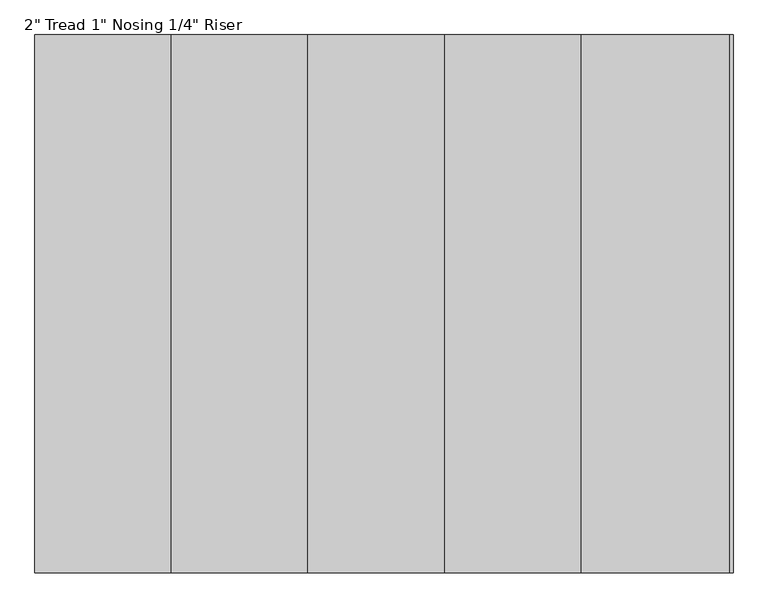
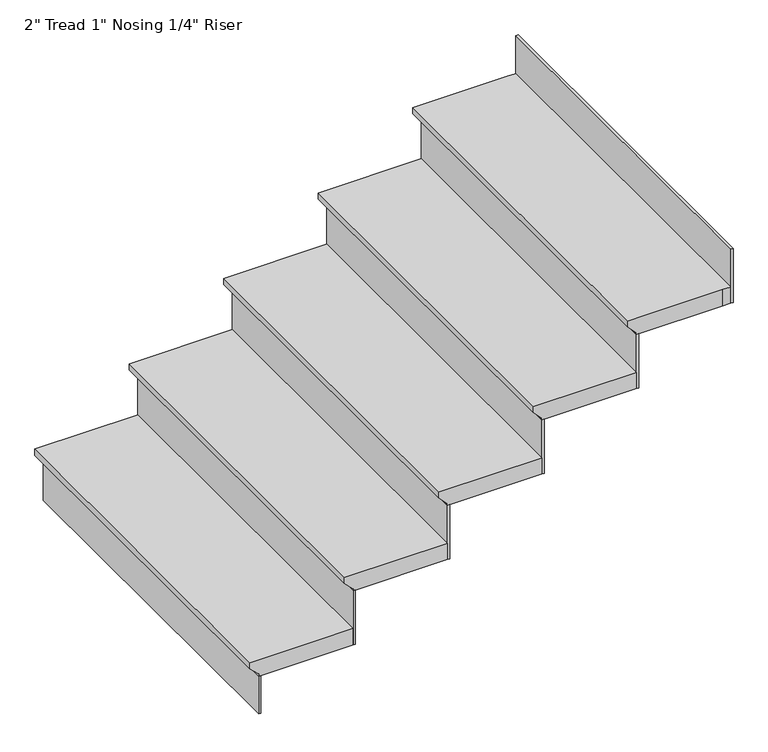
"""IFC4 building model written with IfcOpenShell, lengths in millimetres: stair flight geometry."""

from ifc_helpers import new_model, si_unit, origin, place, context, project, spatial, faceted_brep, source, transform, mapped, element, save


def stair_flight_239b6ec8(model_context):
    return source(origin(), model_context, "Body", "Brep", [
        faceted_brep([(-3170.5888787, 2474.8939653, 150.2833333), (-3170.5888787, 2474.8939653, 169.3333333), (-3170.5888787, 3576.1973029, 169.3333333), (-3170.5888787, 3576.1973029, 150.2833333), (-3145.1888787, 2474.8939653, 124.8833333), (-3145.1888787, 3576.1973029, 124.8833333), (-2865.7888787, 2474.8939653, 169.3333333), (-2865.7888787, 3576.1973029, 169.3333333), (-3145.1888787, 3576.1973029, 118.5333333), (-2865.7888787, 3576.1973029, 118.5333333), (-2865.7888787, 2474.8939653, 118.5333333), (-3145.1888787, 2474.8939653, 118.5333333)], [[[0, 1, 2, 3]], [[4, 0, 3, 5]], [[2, 1, 6, 7]], [[8, 9, 10, 11]], [[2, 7, 9, 8, 5, 3]], [[8, 11, 4, 5]], [[6, 1, 0, 4, 11, 10]], [[7, 6, 10, 9]]]),
        faceted_brep([(-3145.1888787, 2474.8939653, 118.5333333), (-3145.1888787, 2474.8939653, 0.0), (-3138.8388787, 2474.8939653, 0.0), (-3138.8388787, 2474.8939653, 118.5333333), (-3145.1888787, 3576.1973029, 118.5333333), (-3138.8388787, 3576.1973029, 118.5333333), (-3138.8388787, 3576.1973029, 0.0), (-3145.1888787, 3576.1973029, 0.0)], [[[0, 1, 2, 3]], [[4, 5, 6, 7]], [[1, 0, 4, 7]], [[2, 1, 7, 6]], [[3, 2, 6, 5]], [[0, 3, 5, 4]]]),
        faceted_brep([(-2865.7888787, 2474.8939653, 287.8666667), (-2865.7888787, 2474.8939653, 118.5333333), (-2859.4388787, 2474.8939653, 118.5333333), (-2859.4388787, 2474.8939653, 287.8666667), (-2865.7888787, 3576.1973029, 287.8666667), (-2859.4388787, 3576.1973029, 287.8666667), (-2859.4388787, 3576.1973029, 118.5333333), (-2865.7888787, 3576.1973029, 118.5333333)], [[[0, 1, 2, 3]], [[4, 5, 6, 7]], [[1, 0, 4, 7]], [[2, 1, 7, 6]], [[3, 2, 6, 5]], [[0, 3, 5, 4]]]),
        faceted_brep([(-2891.1888787, 3576.1973029, 338.6666667), (-2891.1888787, 2474.8939653, 338.6666667), (-2586.3888787, 2474.8939653, 338.6666667), (-2586.3888787, 3576.1973029, 338.6666667), (-2865.7888787, 3576.1973029, 287.8666667), (-2586.3888787, 3576.1973029, 287.8666667), (-2586.3888787, 2474.8939653, 287.8666667), (-2865.7888787, 2474.8939653, 287.8666667), (-2865.7888787, 3576.1973029, 294.2166667), (-2891.1888787, 3576.1973029, 319.6166667), (-2865.7888787, 2474.8939653, 294.2166667), (-2891.1888787, 2474.8939653, 319.6166667)], [[[0, 1, 2, 3]], [[4, 5, 6, 7]], [[0, 3, 5, 4, 8, 9]], [[4, 7, 10, 8]], [[2, 1, 11, 10, 7, 6]], [[3, 2, 6, 5]], [[11, 1, 0, 9]], [[10, 11, 9, 8]]]),
        faceted_brep([(-2586.3888787, 2474.8939653, 457.2), (-2586.3888787, 2474.8939653, 287.8666667), (-2580.0388787, 2474.8939653, 287.8666667), (-2580.0388787, 2474.8939653, 457.2), (-2586.3888787, 3576.1973029, 457.2), (-2580.0388787, 3576.1973029, 457.2), (-2580.0388787, 3576.1973029, 287.8666667), (-2586.3888787, 3576.1973029, 287.8666667)], [[[0, 1, 2, 3]], [[4, 5, 6, 7]], [[1, 0, 4, 7]], [[2, 1, 7, 6]], [[3, 2, 6, 5]], [[0, 3, 5, 4]]]),
        faceted_brep([(-2611.7888787, 3576.1973029, 508.0), (-2611.7888787, 2474.8939653, 508.0), (-2306.9888787, 2474.8939653, 508.0), (-2306.9888787, 3576.1973029, 508.0), (-2586.3888787, 3576.1973029, 457.2), (-2306.9888787, 3576.1973029, 457.2), (-2306.9888787, 2474.8939653, 457.2), (-2586.3888787, 2474.8939653, 457.2), (-2586.3888787, 3576.1973029, 463.55), (-2611.7888787, 3576.1973029, 488.95), (-2586.3888787, 2474.8939653, 463.55), (-2611.7888787, 2474.8939653, 488.95)], [[[0, 1, 2, 3]], [[4, 5, 6, 7]], [[0, 3, 5, 4, 8, 9]], [[4, 7, 10, 8]], [[2, 1, 11, 10, 7, 6]], [[3, 2, 6, 5]], [[11, 1, 0, 9]], [[10, 11, 9, 8]]]),
        faceted_brep([(-2306.9888787, 2474.8939653, 626.5333333), (-2306.9888787, 2474.8939653, 457.2), (-2300.6388787, 2474.8939653, 457.2), (-2300.6388787, 2474.8939653, 626.5333333), (-2306.9888787, 3576.1973029, 626.5333333), (-2300.6388787, 3576.1973029, 626.5333333), (-2300.6388787, 3576.1973029, 457.2), (-2306.9888787, 3576.1973029, 457.2)], [[[0, 1, 2, 3]], [[4, 5, 6, 7]], [[1, 0, 4, 7]], [[2, 1, 7, 6]], [[3, 2, 6, 5]], [[0, 3, 5, 4]]]),
        faceted_brep([(-2332.3888787, 3576.1973029, 677.3333333), (-2332.3888787, 2474.8939653, 677.3333333), (-2027.5888787, 2474.8939653, 677.3333333), (-2027.5888787, 3576.1973029, 677.3333333), (-2306.9888787, 3576.1973029, 626.5333333), (-2027.5888787, 3576.1973029, 626.5333333), (-2027.5888787, 2474.8939653, 626.5333333), (-2306.9888787, 2474.8939653, 626.5333333), (-2306.9888787, 3576.1973029, 632.8833333), (-2332.3888787, 3576.1973029, 658.2833333), (-2306.9888787, 2474.8939653, 632.8833333), (-2332.3888787, 2474.8939653, 658.2833333)], [[[0, 1, 2, 3]], [[4, 5, 6, 7]], [[0, 3, 5, 4, 8, 9]], [[4, 7, 10, 8]], [[2, 1, 11, 10, 7, 6]], [[3, 2, 6, 5]], [[11, 1, 0, 9]], [[10, 11, 9, 8]]]),
        faceted_brep([(-1748.1888787, 2474.8939653, 965.2), (-1748.1888787, 2474.8939653, 795.8666667), (-1741.8388787, 2474.8939653, 795.8666667), (-1741.8388787, 2474.8939653, 965.2), (-1748.1888787, 3576.1973029, 965.2), (-1741.8388787, 3576.1973029, 965.2), (-1741.8388787, 3576.1973029, 795.8666667), (-1748.1888787, 3576.1973029, 795.8666667)], [[[0, 1, 2, 3]], [[4, 5, 6, 7]], [[1, 0, 4, 7]], [[2, 1, 7, 6]], [[3, 2, 6, 5]], [[0, 3, 5, 4]]]),
        faceted_brep([(-2027.5888787, 2474.8939653, 795.8666667), (-2027.5888787, 2474.8939653, 626.5333333), (-2021.2388787, 2474.8939653, 626.5333333), (-2021.2388787, 2474.8939653, 795.8666667), (-2027.5888787, 3576.1973029, 795.8666667), (-2021.2388787, 3576.1973029, 795.8666667), (-2021.2388787, 3576.1973029, 626.5333333), (-2027.5888787, 3576.1973029, 626.5333333)], [[[0, 1, 2, 3]], [[4, 5, 6, 7]], [[1, 0, 4, 7]], [[2, 1, 7, 6]], [[3, 2, 6, 5]], [[0, 3, 5, 4]]]),
        faceted_brep([(-1748.1888787, 3576.1973029, 846.6666667), (-1773.5888787, 3576.1973029, 846.6666667), (-2052.9888787, 3576.1973029, 846.6666667), (-2052.9888787, 2474.8939653, 846.6666667), (-1773.5888787, 2474.8939653, 846.6666667), (-1748.1888787, 2474.8939653, 846.6666667), (-1773.5888787, 3576.1973029, 795.8666667), (-1748.1888787, 3576.1973029, 795.8666667), (-1748.1888787, 2474.8939653, 795.8666667), (-1773.5888787, 2474.8939653, 795.8666667), (-2027.5888787, 2474.8939653, 795.8666667), (-2027.5888787, 3576.1973029, 795.8666667), (-2027.5888787, 3576.1973029, 802.2166667), (-2052.9888787, 3576.1973029, 827.6166667), (-2027.5888787, 2474.8939653, 802.2166667), (-2052.9888787, 2474.8939653, 827.6166667)], [[[0, 1, 2, 3, 4, 5]], [[6, 7, 8, 9, 10, 11]], [[1, 0, 7, 6]], [[2, 1, 6, 11, 12, 13]], [[11, 10, 14, 12]], [[4, 3, 15, 14, 10, 9]], [[5, 4, 9, 8]], [[0, 5, 8, 7]], [[15, 3, 2, 13]], [[14, 15, 13, 12]]]),
    ])


if __name__ == "__main__":
    model = new_model("IFC4")
    model_context = context("Model", 3, world=origin())
    ifc_project = project(units=[si_unit("LENGTHUNIT", "METRE", prefix="MILLI")], contexts=[model_context])
    site = spatial("IfcSite", under=ifc_project)
    building = spatial("IfcBuilding", under=site)
    placement = place(None, origin())
    stair_flight_shape = stair_flight_239b6ec8(model_context)
    element("IfcStairFlight", 1, ObjectType="2\" Tread 1\" Nosing 1/4\" Riser", at=placement, inside=building, context=model_context, shape_type="MappedRepresentation", body=[
        mapped(stair_flight_shape, transform((0.0, 0.0, 0.0), x_axis=(1.0, 0.0, 0.0), y_axis=(0.0, 1.0, 0.0), z_axis=(0.0, 0.0, 1.0))),
    ])
    save(model, "model.ifc")
